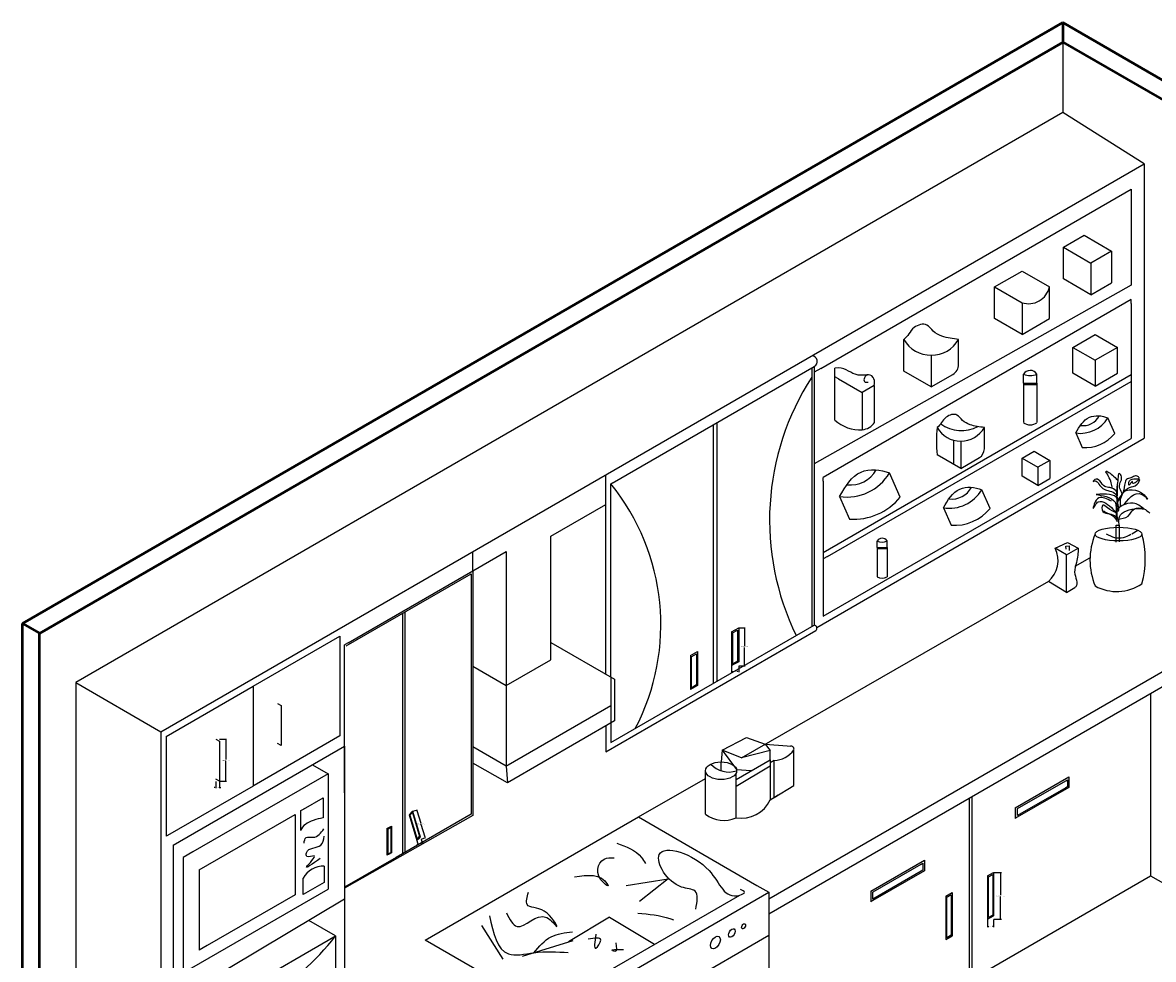
# Model space of a CAD drawing. Units: centimetres. Extents: x 5383 to 11288, y 5305 to 11515.
# Tile 3 of 5: x 5383 to 5675, y 5610 to 5851. Entities that reach past the tile are written whole.
import ezdxf

# ---------------------------------------------------------------- set-up
doc = ezdxf.new("R2010")
doc.units = ezdxf.units.CM
for name, color, linetype, lineweight in [('A-ANNO-DIMS', 2, 'Continuous', 18), ('A-EQPM', 4, 'Continuous', 25), ('A-FLOR-CASE', 3, 'Continuous', 25), ('A-WALL', 7, 'Continuous', 50)]:
    doc.layers.add(name, color=color, linetype=linetype, lineweight=lineweight)
doc.styles.get("Standard").update_dxf_attribs({"font": 'arial.ttf'})
doc.dimstyles.get("Standard").update_dxf_attribs({"dimtxt": 0.18, "dimasz": 0.18, "dimexe": 0.18, "dimexo": 0.0625, "dimgap": 0.09, "dimtad": 0, "dimtih": 1, "dimtoh": 1, "dimdec": 4, "dimzin": 0, "dimdsep": 46, "dimtxsty": 'Standard', "dimcen": 0.09, "dimadec": 0, "dimazin": 0, "dimtfac": 1, "dimtdec": 4, "dimtofl": 0, "dimtmove": 0, "dimatfit": 3, "dimfxl": 1, "dimtolj": 1, "dimtzin": 0, "dimarcsym": 0})

# ---------------------------------------------------------------- blocks, each defined once
blk = doc.blocks.new('HANDLE-DOOR-A')
for p, q in [((0, 8.75), (1.82, 9.8)), ((0.24, 8.46), (1.54, 9.21)), ((1.54, 9.21), (1.54, 1.19)), ((1.82, 9.8), (1.82, 1.05)), ((0, 8.75), (0, 0)), ((0.24, 8.46), (0.24, 0.44)), ((0.49, 0.29), (0, 0)), ((0.33, 0.49), (0.24, 0.44)), ((1.54, 1.19), (0.33, 0.49)), ((1.82, 1.05), (0.49, 0.29))]:
    blk.add_line(p, q)
blk = doc.blocks.new('HANDLE-DOOR-B')
for p, q in [((0, 6.88), (1.13, 7.53)), ((0, 6.88), (0, 0)), ((0.2, 6.74), (0.98, 7.19)), ((0.2, 6.74), (0.2, 0.29)), ((0.98, 7.19), (0.98, 0.75)), ((1.13, 7.53), (1.13, 0.65)), ((0.41, 0.24), (0, 0)), ((0.2, 0.29), (0.98, 0.75)), ((1.13, 0.65), (0.41, 0.24))]:
    blk.add_line(p, q)
blk = doc.blocks.new('HANDLE-DOOR-C')
for p, q in [((0, 11.18), (1.56, 12.08)), ((1.56, 12.08), (1.56, 0.91)), ((0, 11.18), (0, 0)), ((0.24, 10.92), (1.35, 11.56)), ((0.24, 0.46), (0.24, 10.92)), ((1.35, 11.56), (1.35, 1.1)), ((0, 0), (1.56, 0.91)), ((1.35, 1.1), (0.24, 0.46)), ((1.56, 0.91), (0.77, 0.45))]:
    blk.add_line(p, q)
blk = doc.blocks.new('HANDLE-DOOR-F')
for p, q in [((0, 10.85), (0.96, 10.3)), ((0.96, 10.3), (0.96, 0)), ((0.96, 0), (0, 0.55))]:
    blk.add_line(p, q)
blk = doc.blocks.new('*D18')
at = {"layer": 'A-ANNO-DIMS', "color": 0, "lineweight": -2, "transparency": 16777216}
for p, q in [((5567.7, 5695.2), (5569.28, 5695.2)), ((5569.1, 5695.02), (5569.1, 5690.48)), ((5569.1, 5685.57), (5569.1, 5690.11)), ((5567.7, 5685.39), (5569.28, 5685.39))]:
    blk.add_line(p, q, dxfattribs=at)
at = {"layer": 'A-ANNO-DIMS', "color": 0, "transparency": 16777216}
for points in [[(5569.07, 5695.02), (5569.13, 5695.02), (5569.1, 5695.2)], [(5569.07, 5685.57), (5569.13, 5685.57), (5569.1, 5685.39)]]:
    blk.add_solid(points, dxfattribs=at)
at = {"layer": 'Defpoints', "color": 0, "transparency": 16777216}
for p in [(5567.63, 5695.2), (5569.1, 5695.2), (5567.63, 5685.39)]:
    blk.add_point(p, dxfattribs=at)
at = {"layer": 'A-ANNO-DIMS', "color": 0, "transparency": 16777216, "insert": (5569.1, 5690.29), "char_height": 0.18, "attachment_point": 5}
blk.add_mtext('\\A1;HANDLE A 10 TYP.', dxfattribs=at)
blk = doc.blocks.new('*D19')
at = {"layer": 'A-ANNO-DIMS', "color": 0, "lineweight": -2, "transparency": 16777216}
for p, q in [((5565.81, 5685.33), (5565.81, 5683.74)), ((5567.63, 5685.33), (5567.63, 5683.74)), ((5565.99, 5683.92), (5566.26, 5683.92)), ((5567.45, 5683.92), (5567.18, 5683.92))]:
    blk.add_line(p, q, dxfattribs=at)
at = {"layer": 'A-ANNO-DIMS', "color": 0, "transparency": 16777216}
for points in [[(5565.99, 5683.95), (5565.99, 5683.89), (5565.81, 5683.92)], [(5567.45, 5683.95), (5567.45, 5683.89), (5567.63, 5683.92)]]:
    blk.add_solid(points, dxfattribs=at)
at = {"layer": 'Defpoints', "color": 0, "transparency": 16777216}
for p in [(5565.81, 5685.39), (5567.63, 5685.39), (5567.63, 5683.92)]:
    blk.add_point(p, dxfattribs=at)
at = {"layer": 'A-ANNO-DIMS', "color": 0, "transparency": 16777216, "insert": (5566.72, 5683.92), "char_height": 0.18, "attachment_point": 5}
blk.add_mtext('\\A1;2 TYP.', dxfattribs=at)
blk = doc.blocks.new('*D20')
at = {"layer": 'A-ANNO-DIMS', "color": 0, "lineweight": -2, "transparency": 16777216}
for p, q in [((5483.53, 5647.9), (5484.72, 5648.26)), ((5484.6, 5648.03), (5485.59, 5644.78)), ((5486.68, 5641.17), (5485.7, 5644.42)), ((5485.71, 5640.69), (5486.91, 5641.05))]:
    blk.add_line(p, q, dxfattribs=at)
at = {"layer": 'A-ANNO-DIMS', "color": 0, "transparency": 16777216}
for points in [[(5484.63, 5648.04), (5484.57, 5648.03), (5484.55, 5648.21)], [(5486.71, 5641.18), (5486.65, 5641.16), (5486.74, 5641)]]:
    blk.add_solid(points, dxfattribs=at)
at = {"layer": 'Defpoints', "color": 0, "transparency": 16777216}
for p in [(5483.47, 5647.88), (5484.55, 5648.21), (5485.65, 5640.67)]:
    blk.add_point(p, dxfattribs=at)
at = {"layer": 'A-ANNO-DIMS', "color": 0, "transparency": 16777216, "insert": (5485.64, 5644.6), "char_height": 0.18, "attachment_point": 5}
blk.add_mtext('\\A1;HANDLE B 8 TYP.', dxfattribs=at)
blk = doc.blocks.new('*D21')
at = {"layer": 'A-ANNO-DIMS', "color": 0, "lineweight": -2, "transparency": 16777216}
for p, q in [((5484.73, 5639.21), (5484.55, 5639.15)), ((5484.59, 5640.28), (5484.95, 5639.09)), ((5485.67, 5640.61), (5486.03, 5639.41)), ((5486.15, 5639.64), (5486.33, 5639.69))]:
    blk.add_line(p, q, dxfattribs=at)
at = {"layer": 'A-ANNO-DIMS', "color": 0, "transparency": 16777216}
for points in [[(5484.72, 5639.23), (5484.73, 5639.18), (5484.9, 5639.26)], [(5486.15, 5639.67), (5486.16, 5639.61), (5485.98, 5639.59)]]:
    blk.add_solid(points, dxfattribs=at)
at = {"layer": 'Defpoints', "color": 0, "transparency": 16777216}
for p in [(5484.57, 5640.34), (5485.65, 5640.67), (5485.98, 5639.59)]:
    blk.add_point(p, dxfattribs=at)
at = {"layer": 'A-ANNO-DIMS', "color": 0, "transparency": 16777216, "insert": (5485.44, 5639.42), "char_height": 0.18, "attachment_point": 5}
blk.add_mtext('\\A1;1 TYP.', dxfattribs=at)
blk = doc.blocks.new('*D22')
at = {"layer": 'A-ANNO-DIMS', "color": 0, "lineweight": -2, "transparency": 16777216}
for p, q in [((5633.49, 5632.05), (5635.42, 5632.05)), ((5635.24, 5631.87), (5635.24, 5626.2)), ((5635.24, 5620.16), (5635.24, 5625.83)), ((5633.49, 5619.98), (5635.42, 5619.98))]:
    blk.add_line(p, q, dxfattribs=at)
at = {"layer": 'A-ANNO-DIMS', "color": 0, "transparency": 16777216}
for points in [[(5635.21, 5631.87), (5635.27, 5631.87), (5635.24, 5632.05)], [(5635.21, 5620.16), (5635.27, 5620.16), (5635.24, 5619.98)]]:
    blk.add_solid(points, dxfattribs=at)
at = {"layer": 'Defpoints', "color": 0, "transparency": 16777216}
for p in [(5633.43, 5632.05), (5635.24, 5632.05), (5633.43, 5619.98)]:
    blk.add_point(p, dxfattribs=at)
at = {"layer": 'A-ANNO-DIMS', "color": 0, "transparency": 16777216, "insert": (5635.24, 5626.01), "char_height": 0.18, "attachment_point": 5}
blk.add_mtext('\\A1;HANDLE C 12 TYP.', dxfattribs=at)
blk = doc.blocks.new('*D23')
at = {"layer": 'A-ANNO-DIMS', "color": 0, "lineweight": -2, "transparency": 16777216}
for p, q in [((5631.87, 5619.91), (5631.87, 5617.98)), ((5632.05, 5618.16), (5632.19, 5618.16)), ((5633.25, 5618.16), (5633.11, 5618.16)), ((5633.43, 5619.91), (5633.43, 5617.98))]:
    blk.add_line(p, q, dxfattribs=at)
at = {"layer": 'A-ANNO-DIMS', "color": 0, "transparency": 16777216}
for points in [[(5632.05, 5618.19), (5632.05, 5618.13), (5631.87, 5618.16)], [(5633.25, 5618.19), (5633.25, 5618.13), (5633.43, 5618.16)]]:
    blk.add_solid(points, dxfattribs=at)
at = {"layer": 'Defpoints', "color": 0, "transparency": 16777216}
for p in [(5631.87, 5619.98), (5633.43, 5619.98), (5633.43, 5618.16)]:
    blk.add_point(p, dxfattribs=at)
at = {"layer": 'A-ANNO-DIMS', "color": 0, "transparency": 16777216, "insert": (5632.65, 5618.16), "char_height": 0.18, "attachment_point": 5}
blk.add_mtext('\\A1;2 TYP.', dxfattribs=at)
blk = doc.blocks.new('*D30')
at = {"layer": 'A-ANNO-DIMS', "color": 0, "lineweight": -2, "transparency": 16777216}
for p, q in [((5433.68, 5666.45), (5435.42, 5666.45)), ((5435.24, 5666.27), (5435.24, 5661.2)), ((5435.24, 5655.77), (5435.24, 5660.84)), ((5433.68, 5655.59), (5435.42, 5655.59))]:
    blk.add_line(p, q, dxfattribs=at)
at = {"layer": 'A-ANNO-DIMS', "color": 0, "transparency": 16777216}
for points in [[(5435.21, 5666.27), (5435.27, 5666.27), (5435.24, 5666.45)], [(5435.21, 5655.77), (5435.27, 5655.77), (5435.24, 5655.59)]]:
    blk.add_solid(points, dxfattribs=at)
at = {"layer": 'Defpoints', "color": 0, "transparency": 16777216}
for p in [(5433.61, 5666.45), (5435.24, 5666.45), (5433.61, 5655.59)]:
    blk.add_point(p, dxfattribs=at)
at = {"layer": 'A-ANNO-DIMS', "color": 0, "transparency": 16777216, "insert": (5435.24, 5661.02), "char_height": 0.18, "attachment_point": 5}
blk.add_mtext('\\A1;HANDLE F 11 TYP.', dxfattribs=at)
blk = doc.blocks.new('*D31')
at = {"layer": 'A-ANNO-DIMS', "color": 0, "lineweight": -2, "transparency": 16777216}
for p, q in [((5432.48, 5653.97), (5432.3, 5653.97)), ((5432.66, 5655.53), (5432.66, 5653.79)), ((5433.61, 5655.53), (5433.61, 5653.79)), ((5433.79, 5653.97), (5433.97, 5653.97))]:
    blk.add_line(p, q, dxfattribs=at)
at = {"layer": 'A-ANNO-DIMS', "color": 0, "transparency": 16777216}
for points in [[(5432.48, 5654), (5432.48, 5653.94), (5432.66, 5653.97)], [(5433.79, 5654), (5433.79, 5653.94), (5433.61, 5653.97)]]:
    blk.add_solid(points, dxfattribs=at)
at = {"layer": 'Defpoints', "color": 0, "transparency": 16777216}
for p in [(5432.66, 5655.59), (5433.61, 5655.59), (5433.61, 5653.97)]:
    blk.add_point(p, dxfattribs=at)
at = {"layer": 'A-ANNO-DIMS', "color": 0, "transparency": 16777216, "insert": (5433.14, 5653.97), "char_height": 0.18, "attachment_point": 5}
blk.add_mtext('\\A1;1 TYP.', dxfattribs=at)

msp = doc.modelspace()

# ---------------------------------------------------------------- linework, layer by layer
at = {"layer": 'A-EQPM'}
for p, q in [((5533.38, 5683.19), (5533.38, 5734.67)), ((5519.18, 5718.86), (5533.38, 5727.01)), ((5519.18, 5686.95), (5519.18, 5718.86)), ((5499.05, 5685.25), (5507.64, 5680.29)), ((5507.64, 5680.29), (5519.18, 5686.95)), ((5457.63, 5659.86), (5461.66, 5657.53)), ((5461.66, 5657.53), (5426.73, 5637.37)), ((5461.66, 5657.53), (5461.66, 5627.75)), ((5541.77, 5646.4), (5559.1, 5656.34)), ((5455.31, 5648.43), (5460.36, 5651.35)), ((5460.36, 5651.35), (5460.36, 5646.17)), ((5428.43, 5632.72), (5453.15, 5647)), ((5453.15, 5647), (5453.15, 5626.31)), ((5454.67, 5648.08), (5455.89, 5648.77)), ((5454.67, 5642.89), (5454.67, 5648.08)), ((5486.72, 5614.62), (5541.77, 5646.4)), ((5541.77, 5646.4), (5572.35, 5628.74)), ((5426.73, 5637.37), (5424.24, 5635.93)), ((5424.24, 5635.93), (5424.24, 5606.15)), ((5428.43, 5632.72), (5428.43, 5612.23)), ((5460.68, 5633.67), (5460.68, 5629.48)), ((5455.24, 5626.34), (5455.24, 5630.57)), ((5460.68, 5629.48), (5455.24, 5626.34)), ((5538.63, 5628.74), (5549.42, 5630.41)), ((5549.42, 5630.41), (5542.07, 5624.55)), ((5424.24, 5606.15), (5461.66, 5627.75)), ((5520.4, 5595.18), (5575.44, 5626.96)), ((5572.35, 5628.74), (5575.44, 5626.96)), ((5575.44, 5626.96), (5575.44, 5615.8)), ((5465.93, 5625.19), (5424.24, 5600.32)), ((5453.15, 5626.31), (5430.43, 5613.2)), ((5520.3, 5598.74), (5567.93, 5626.24)), ((5501.25, 5618.39), (5506.79, 5609.7)), ((5534.29, 5620.52), (5523.7, 5614.15)), ((5534.29, 5620.52), (5545.94, 5613.54)), ((5575.44, 5615.8), (5520.4, 5584.02)), ((5575.44, 5615.8), (5575.44, 5574.33)), ((5430.43, 5613.2), (5428.43, 5612.04)), ((5428.43, 5612.23), (5428.43, 5612.04)), ((5520.4, 5595.18), (5486.72, 5614.62)), ((5511.85, 5610.43), (5524.88, 5614.52))]:
    msp.add_line(p, q, dxfattribs=at)
msp.add_arc((5460.45, 5627.75), 5.93, 87.7657, 151.5311, dxfattribs=at)
for centre, major_axis in [((5565.87, 5616.43), (-0.61, -1.05)), ((5568.89, 5618.17), (-0.368, -0.638)), ((5561.63, 5613.98), (-0.9, -1.55))]:
    msp.add_ellipse(centre, major_axis=major_axis, ratio=0.57735, dxfattribs=at)
for points, knots in [([(5460.36, 5646.17), (5459.55, 5645.98), (5457.46, 5645.48), (5454.9, 5644.17), (5454.67, 5642.89)], [0, 0, 0, 0, 2.608233, 6.700151, 6.700151, 6.700151, 6.700151]), ([(5455.46, 5639.64), (5455.55, 5640.23), (5455.74, 5641.55), (5458.64, 5640.66), (5459.81, 5642.24), (5460.58, 5643.29)], [0, 0, 0, 0, 1.518182, 3.345478, 6.853378, 6.853378, 6.853378, 6.853378]), ([(5459.63, 5635.68), (5457.66, 5634.26), (5454.08, 5631.68), (5459.75, 5637.33), (5456.02, 5635.56), (5455.97, 5638.7), (5460.16, 5638.07), (5460.53, 5640.51), (5460.66, 5641.39)], [0, 0, 0, 0, 4.047225, 7.363085, 9.194771, 10.155201, 14.385132, 16.797476, 16.797476, 16.797476, 16.797476]), ([(5536.16, 5639.64), (5538.6, 5638.74), (5541.66, 5637.6), (5543.28, 5634.92), (5543.61, 5634.37)], [0, 0, 0, 0, 7.386801, 9.288551, 9.288551, 9.288551, 9.288551]), ([(5556.55, 5622.59), (5556.9, 5624.51), (5557.53, 5627.95), (5550.15, 5627.71), (5542.48, 5641.3), (5561.88, 5634.99), (5563.87, 5624.44), (5569.7, 5626.92), (5568.59, 5627.4), (5568.06, 5627.63)], [0, 0, 0, 0, 4.660279, 8.330693, 18.454163, 31.926211, 42.090752, 43.472118, 44.746413, 44.746413, 44.746413, 44.746413]), ([(5525.26, 5630.95), (5528.64, 5631.44), (5532.15, 5631.95), (5534.19, 5628.29), (5530.22, 5630.93), (5531.43, 5635.96), (5534.57, 5635.86), (5535.49, 5635.83)], [0, 0, 0, 0, 8.778444, 9.119705, 10.35063, 16.607257, 19.221094, 19.221094, 19.221094, 19.221094]), ([(5507.7, 5621.64), (5508.52, 5620), (5510.81, 5615.44), (5516.6, 5623.49), (5522.14, 5615.93), (5517.91, 5623.64), (5512.18, 5622.55), (5513.01, 5625.7), (5513.35, 5626.98)], [0, 0, 0, 0, 4.458018, 12.428882, 15.889863, 20.991355, 25.727205, 28.946338, 28.946338, 28.946338, 28.946338]), ([(5503.3, 5620.84), (5504.28, 5616.44), (5505.84, 5609.41), (5515.77, 5611.86), (5520.76, 5611.59), (5523.63, 5611.43)], [0, 0, 0, 0, 10.970099, 17.518453, 26.404777, 26.404777, 26.404777, 26.404777]), ([(5541.63, 5621.58), (5544.43, 5621.32), (5547.56, 5621.02), (5550.49, 5619.94), (5550.79, 5619.83)], [0, 0, 0, 0, 8.376196, 9.342218, 9.342218, 9.342218, 9.342218]), ([(5514.75, 5611.34), (5516.12, 5612.94), (5518.76, 5616.03), (5522.79, 5616.51), (5524.73, 5616.74)], [0, 0, 0, 0, 6.070874, 11.732161, 11.732161, 11.732161, 11.732161]), ([(5530.79, 5616.12), (5530.48, 5614.19), (5529.95, 5610.97), (5533.21, 5615.63), (5530.4, 5615.15), (5528.77, 5614.87)], [0, 0, 0, 0, 3.555518, 5.929323, 9.211396, 9.211396, 9.211396, 9.211396]), ([(5535.89, 5613.88), (5536.13, 5612.78), (5536.44, 5611.35), (5534.05, 5612.23), (5536.17, 5612.2), (5537.9, 5612.17)], [0, 0, 0, 0, 2.20234, 2.83923, 5.661966, 5.661966, 5.661966, 5.661966])]:
    msp.add_open_spline(points, degree=3, knots=knots, dxfattribs=at)
at = {"layer": 'A-FLOR-CASE'}
for p, q in [((5651.3, 5846.21), (5651.3, 5828.15)), ((5651.3, 5828.15), (5396.53, 5681.06)), ((5672.32, 5814.89), (5651.3, 5828.15)), ((5418.53, 5668.36), (5672.32, 5814.89)), ((5672.32, 5814.89), (5672.32, 5744.1)), ((5588.84, 5762.08), (5668.92, 5808.32)), ((5668.92, 5808.32), (5668.92, 5783.56)), ((5651.42, 5793.36), (5656.79, 5796.47)), ((5656.78, 5796.47), (5663.86, 5792.39)), ((5651.42, 5785.19), (5651.42, 5793.36)), ((5651.42, 5793.36), (5658.49, 5789.28)), ((5663.87, 5792.38), (5658.49, 5789.28)), ((5663.86, 5792.39), (5663.87, 5792.38)), ((5663.87, 5792.38), (5663.87, 5784.21)), ((5633.69, 5783.13), (5640.76, 5787.21)), ((5640.76, 5787.21), (5647.84, 5783.13)), ((5658.49, 5789.28), (5658.49, 5781.11)), ((5658.49, 5781.11), (5651.42, 5785.19)), ((5658.49, 5781.11), (5663.87, 5784.21)), ((5668.92, 5783.56), (5587.15, 5737.46)), ((5633.69, 5774.96), (5633.69, 5783.13)), ((5633.69, 5783.13), (5640.76, 5779.04)), ((5647.84, 5774.96), (5647.84, 5783.13)), ((5668.92, 5779.91), (5589.43, 5734.01)), ((5640.76, 5779.04), (5640.76, 5770.87)), ((5668.92, 5778.88), (5668.92, 5779.91)), ((5668.92, 5778.88), (5668.92, 5760.43)), ((5640.76, 5770.87), (5633.69, 5774.96)), ((5640.76, 5770.87), (5647.84, 5774.96)), ((5610.24, 5761.42), (5610.24, 5769.59)), ((5624.4, 5763.15), (5624.4, 5769.59)), ((5653.91, 5767.52), (5659.66, 5770.84)), ((5659.66, 5770.84), (5665.41, 5767.52)), ((5653.91, 5760.88), (5653.91, 5767.52)), ((5653.91, 5767.52), (5659.66, 5764.2)), ((5665.41, 5767.52), (5659.66, 5764.2)), ((5665.41, 5760.88), (5665.41, 5767.52)), ((5617.32, 5765.51), (5617.32, 5757.33)), ((5659.66, 5764.2), (5659.66, 5757.57)), ((5535.01, 5732.54), (5587.15, 5762.65)), ((5586.52, 5762.28), (5586.52, 5695.51)), ((5587.15, 5762.65), (5587.15, 5695.88)), ((5588.84, 5762.08), (5587.15, 5761.11)), ((5592.48, 5748.74), (5592.48, 5762.17)), ((5617.32, 5757.33), (5610.24, 5761.42)), ((5644.62, 5758.32), (5644.62, 5760.67)), ((5659.66, 5757.57), (5653.91, 5760.88)), ((5659.66, 5757.57), (5665.41, 5760.88)), ((5668.92, 5760.43), (5589.43, 5714.53)), ((5590.52, 5713.61), (5668.92, 5758.75)), ((5593.39, 5759.41), (5592.48, 5759.93)), ((5593.39, 5759.41), (5599.52, 5755.93)), ((5617.32, 5757.33), (5622.9, 5760.55)), ((5641.11, 5758.32), (5641.11, 5760.61)), ((5641.11, 5758.32), (5641.11, 5748.12)), ((5641.11, 5758.32), (5644.62, 5758.32)), ((5641.11, 5758), (5644.62, 5758)), ((5644.62, 5758.32), (5644.62, 5748.12)), ((5668.92, 5760.43), (5668.92, 5744.07)), ((5602.58, 5757.7), (5599.52, 5755.93)), ((5599.52, 5755.93), (5599.52, 5746.29)), ((5602.71, 5748.16), (5602.71, 5757.7)), ((5664.7, 5745.34), (5662.92, 5749.38)), ((5561.08, 5747.6), (5561.08, 5680.83)), ((5561.98, 5748.12), (5561.98, 5681.35)), ((5631.04, 5741.33), (5631.04, 5746.87)), ((5587.77, 5695.29), (5672.32, 5744.1)), ((5589.43, 5698.17), (5668.92, 5744.07)), ((5623.11, 5743.6), (5623.11, 5737.37)), ((5624.94, 5743.35), (5624.94, 5736.31)), ((5654.61, 5745.45), (5656.27, 5741.69)), ((5640.78, 5738.95), (5643.85, 5740.72)), ((5643.85, 5740.72), (5647.9, 5738.39)), ((5624.94, 5736.31), (5618.85, 5739.83)), ((5624.94, 5736.31), (5629.75, 5739.09)), ((5640.78, 5734.27), (5640.78, 5738.95)), ((5640.78, 5738.95), (5644.83, 5736.61)), ((5647.9, 5738.38), (5644.83, 5736.61)), ((5647.9, 5738.38), (5647.9, 5733.71)), ((5609.34, 5728.9), (5606.58, 5735.16)), ((5644.83, 5736.61), (5644.83, 5731.94)), ((5535.01, 5732.54), (5534.64, 5732.33)), ((5534.64, 5730.09), (5534.64, 5732.33)), ((5589.43, 5732.98), (5589.43, 5734.01)), ((5589.43, 5732.98), (5589.43, 5698.17)), ((5644.83, 5731.94), (5640.78, 5734.27)), ((5644.83, 5731.94), (5647.9, 5733.71)), ((5665.32, 5722.65), (5665.32, 5731.74)), ((5534.64, 5682.45), (5534.64, 5730.09)), ((5593.68, 5729.07), (5596.26, 5723.24)), ((5632.5, 5726), (5630.38, 5730.82)), ((5620.45, 5726.14), (5622.44, 5721.64)), ((5665.04, 5717.29), (5665.04, 5721.65)), ((5665.04, 5721.65), (5665.95, 5721.65)), ((5665.95, 5717.35), (5665.95, 5721.65)), ((5669.07, 5719.45), (5670.67, 5720.37)), ((5603.34, 5715.92), (5603.34, 5717.61)), ((5605.93, 5715.89), (5605.93, 5717.61)), ((5649.34, 5715.7), (5652.5, 5717.18)), ((5652.5, 5717.18), (5655.25, 5715.75)), ((5499.05, 5709.91), (5507.64, 5714.88)), ((5499.05, 5709.91), (5499.05, 5714.85)), ((5507.64, 5714.88), (5507.64, 5669.22)), ((5603.36, 5715.89), (5603.36, 5708.38)), ((5603.36, 5715.89), (5605.93, 5715.89)), ((5603.36, 5715.65), (5605.93, 5715.65)), ((5605.93, 5715.89), (5605.93, 5708.38)), ((5652.25, 5714.02), (5649.34, 5715.7)), ((5652.04, 5716.28), (5652.92, 5716.35)), ((5652.11, 5715.47), (5652.04, 5716.28)), ((5652.25, 5714.02), (5655.25, 5715.75)), ((5652.25, 5704.32), (5652.25, 5714.02)), ((5652.92, 5716.35), (5652.92, 5715.12)), ((5590.52, 5713.61), (5589.43, 5712.97)), ((5654.5, 5711.09), (5658.29, 5713.27)), ((5466.33, 5690.51), (5498.59, 5709.14)), ((5466.82, 5691.3), (5499.05, 5709.91)), ((5498.59, 5709.14), (5498.59, 5647.1)), ((5499.05, 5709.91), (5499.05, 5646.79)), ((5568.34, 5661.65), (5647.69, 5707.18)), ((5652.25, 5704.32), (5647.57, 5707.13)), ((5652.25, 5704.32), (5654.39, 5705.55)), ((5480.84, 5698.89), (5480.84, 5636.85)), ((5481.5, 5699.27), (5481.5, 5637.23)), ((5533.38, 5663.18), (5587.57, 5694.46)), ((5534.64, 5665.56), (5587.15, 5695.88)), ((5442.33, 5680.13), (5464.69, 5693.05)), ((5464.69, 5693.05), (5464.69, 5667.28)), ((5466.82, 5691.3), (5465.93, 5690.79)), ((5465.93, 5690.43), (5465.93, 5690.79)), ((5519.18, 5691.38), (5535.6, 5681.9)), ((5465.93, 5687.71), (5465.93, 5690.43)), ((5465.93, 5652.59), (5465.93, 5687.71)), ((5575.44, 5625.3), (5678.79, 5684.97)), ((5534.64, 5682.45), (5534.64, 5665.56)), ((5535.6, 5681.9), (5535.6, 5675.63)), ((5396.53, 5681.06), (5396.53, 5496.36)), ((5396.53, 5681.06), (5418.53, 5668.36)), ((5419.92, 5667.17), (5442.29, 5680.09)), ((5442.29, 5680.09), (5442.29, 5654.32)), ((5442.33, 5680.13), (5442.33, 5654.37)), ((5575.44, 5621.38), (5678.79, 5681.05)), ((5673.95, 5678.25), (5673.95, 5631.2)), ((5534.64, 5675.07), (5508.13, 5659.77)), ((5535.6, 5675.63), (5535.6, 5671.17)), ((5535.6, 5671.17), (5507.93, 5655.19)), ((5418.53, 5668.36), (5418.53, 5504.61)), ((5464.69, 5667.28), (5442.61, 5654.53)), ((5507.64, 5669.22), (5507.64, 5659.48)), ((5533.38, 5669.88), (5533.38, 5663.18)), ((5419.92, 5667.17), (5419.92, 5641.41)), ((5421.66, 5639.1), (5465.93, 5664.66)), ((5465.93, 5664.66), (5465.93, 5511.54)), ((5507.64, 5659.48), (5499.05, 5664.45)), ((5563.37, 5663.6), (5569.64, 5666.91)), ((5569.64, 5666.91), (5574.47, 5665.17)), ((5574.47, 5665.17), (5575.77, 5663.5)), ((5574.47, 5665.17), (5580.17, 5664.7)), ((5580.17, 5664.7), (5580.98, 5664.63)), ((5563.37, 5663.6), (5563.1, 5660.59)), ((5568.34, 5661.65), (5563.37, 5663.6)), ((5563.37, 5663.6), (5567.07, 5658.61)), ((5575.77, 5663.5), (5568.34, 5661.65)), ((5575.77, 5661.16), (5575.77, 5663.5)), ((5575.77, 5663.5), (5575.77, 5663.5)), ((5581.88, 5654.5), (5581.88, 5663.7)), ((5507.93, 5655.19), (5499.05, 5660.27)), ((5508.13, 5659.77), (5507.64, 5659.48)), ((5507.64, 5659.48), (5507.93, 5655.19)), ((5563.1, 5658.31), (5563.1, 5660.59)), ((5565.6, 5660.07), (5565.61, 5660.08)), ((5566.96, 5656.07), (5575.77, 5661.16)), ((5575.77, 5659.46), (5566.96, 5654.22)), ((5567.07, 5658.61), (5570.89, 5658.34)), ((5575.77, 5661.16), (5575.77, 5659.46)), ((5576.79, 5660.92), (5575.77, 5660.31)), ((5575.77, 5659.46), (5575.77, 5650.81)), ((5576.79, 5651.43), (5576.79, 5660.92)), ((5559.1, 5654.15), (5559.1, 5658.2)), ((5566.96, 5646.18), (5566.96, 5657.69)), ((5638.98, 5648.74), (5652.83, 5656.73)), ((5639.63, 5648.55), (5652.02, 5655.7)), ((5652.02, 5655.7), (5652.47, 5655.96)), ((5652.47, 5655.96), (5652.47, 5654.18)), ((5652.83, 5656.73), (5652.83, 5654)), ((5442.29, 5654.32), (5420.2, 5641.57)), ((5442.61, 5654.53), (5442.29, 5654.32)), ((5559.1, 5647.14), (5559.1, 5654.15)), ((5576.79, 5651.43), (5581.88, 5654.5)), ((5652.83, 5654), (5639.54, 5646.33)), ((5652.02, 5653.92), (5639.56, 5646.72)), ((5652.47, 5654.18), (5652.02, 5653.92)), ((5575.77, 5650.81), (5577.82, 5652.05)), ((5627.11, 5651.21), (5627.11, 5604.16)), ((5627.78, 5651.6), (5627.78, 5604.55)), ((5498.59, 5647.1), (5479.26, 5635.94)), ((5638.98, 5648.74), (5638.98, 5646.01)), ((5639.56, 5646.72), (5639.56, 5648.51)), ((5499.05, 5646.79), (5465.93, 5628.03)), ((5639.54, 5646.33), (5638.98, 5646.01)), ((5420.2, 5641.57), (5419.92, 5641.41)), ((5421.66, 5639.1), (5421.66, 5485.47)), ((5479.26, 5635.94), (5465.93, 5628.25)), ((5601.71, 5627.22), (5615.55, 5635.21)), ((5615.55, 5635.21), (5615.55, 5632.48)), ((5615.55, 5632.48), (5602.27, 5624.81)), ((5614.74, 5632.4), (5602.29, 5625.2)), ((5602.35, 5627.03), (5614.74, 5634.18)), ((5614.74, 5634.18), (5615.19, 5634.44)), ((5615.19, 5632.65), (5614.74, 5632.4)), ((5615.19, 5634.44), (5615.19, 5632.65)), ((5558.33, 5564.45), (5673.95, 5631.2)), ((5673.95, 5631.2), (5736.51, 5595.08)), ((5601.71, 5627.22), (5601.71, 5624.49)), ((5602.35, 5627.03), (5602.29, 5626.99)), ((5602.29, 5625.2), (5602.29, 5626.99)), ((5602.27, 5624.81), (5601.71, 5624.49)), ((5463.6, 5615.69), (5456.7, 5619.68)), ((5461.72, 5614.61), (5463.6, 5615.69)), ((5463.6, 5615.69), (5463.6, 5518.14)), ((5421.66, 5591.48), (5461.72, 5614.61))]:
    msp.add_line(p, q, dxfattribs=at)
for centre, radius, start, end in [((5642.41, 5784.36), 5.56, 252.7563, 347.2437), ((5617.32, 5773.68), 8.17, 210, 330), ((5586.43, 5763.93), 1.47, 299.3685, 84.2474), ((5621.4, 5763.15), 3, 300, 0), ((5642.88, 5759.53), 2.07, 33.2806, 148.588), ((5642.8, 5764.51), 4.25, 246.6072, 295.2614), ((5643.44, 5722.98), 67.84, 147.0474, 206.05), ((5655.84, 5753.61), 8.25, 261.3996, 329.1091), ((5656.51, 5752.1), 4.74, 261.8793, 332.0456), ((5598.95, 5756.04), 9.76, 228.4196, 273.3124), ((5599.15, 5750.59), 4.31, 274.8828, 325.6975), ((5650.2, 5743.35), 31.55, 173.5951, 186.4049), ((5624.94, 5750.39), 7.04, 210, 330), ((5625.17, 5755.01), 8.97, 233.0487, 298.0753), ((5642.86, 5750.61), 3.05, 234.9464, 305.0536), ((5656.95, 5751.69), 10.02, 266.1295, 320.698), ((5628.45, 5741.33), 2.58, 300, 0), ((5595.59, 5741.73), 12.8, 261.3996, 329.1091), ((5596.62, 5739.39), 7.35, 261.8793, 332.0456), ((5489.88, 5695.98), 57.67, 332.3397, 39.0788), ((5597.3, 5738.75), 15.55, 266.1295, 320.698), ((5621.93, 5735.87), 9.85, 261.3996, 329.1091), ((5622.71, 5734.07), 5.65, 261.8793, 332.0456), ((5623.24, 5733.58), 11.96, 266.1295, 320.698), ((5604.66, 5716.77), 1.52, 33.2806, 148.588), ((5604.6, 5720.44), 3.13, 246.6072, 295.2614), ((5675.57, 5712.68), 17.28, 157.2197, 202.7803), ((5647.6, 5712.96), 24.95, 345.1121, 14.8879), ((5642.82, 5712.58), 7.23, 311.0571, 25.5985), ((5604.64, 5710.21), 2.24, 234.9464, 305.0536), ((5665.21, 5716.12), 11.57, 241.172, 304.1782), ((5586.95, 5695.05), 0.852, 316.2625, 76.2625), ((5426.4, 5631.7), 40.5, 66.8388, 66.9018), ((5581.17, 5663.91), 0.745, 343.4856, 104.3086), ((5576.44, 5667.62), 6.71, 273.0044, 324.1801), ((5565.07, 5664.27), 6.3, 222.5539, 288.8818), ((5568.38, 5654.19), 8.13, 259.939, 335.4526), ((5563.78, 5652.86), 7.39, 230.6657, 295.4474), ((5413.21, 5654.54), 63.63, 277.6292, 322.3708)]:
    msp.add_arc(centre, radius, start, end, dxfattribs=at)
for centre, major_axis, ratio in [((5665.67, 5719.37), (-6.04, 0), 0.292852), ((5563.1, 5658.31), (-4.01, 0), 0.569076)]:
    msp.add_ellipse(centre, major_axis=major_axis, ratio=ratio, dxfattribs=at)
for points, knots in [([(5624.4, 5769.59), (5622.94, 5769.77), (5620.61, 5770.04), (5617.79, 5771.47), (5616.2, 5774.03), (5612.17, 5772.94), (5611.31, 5770.29), (5610.24, 5769.59)], [0, 0, 0, 0, 4.38311, 6.972047, 9.273965, 12.593909, 16.675124, 16.675124, 16.675124, 16.675124]), ([(5600.87, 5760.41), (5599.79, 5760.34), (5597.07, 5760.14), (5594.76, 5762.58), (5592.48, 5762.17)], [0, 0, 0, 0, 2.115163, 5.365679, 5.365679, 5.365679, 5.365679]), ([(5602.58, 5757.7), (5602.68, 5758.28), (5602.88, 5759.46), (5601.26, 5760.91), (5599.96, 5759.91), (5599.87, 5758.47), (5600.67, 5758.53), (5601.09, 5758.56)], [0, 0, 0, 0, 1.692298, 3.480179, 4.827654, 5.771982, 6.812324, 6.812324, 6.812324, 6.812324]), ([(5631.04, 5746.87), (5629.78, 5747.02), (5627.78, 5747.26), (5625.35, 5748.49), (5623.98, 5750.7), (5620.51, 5749.76), (5619.76, 5747.48), (5618.85, 5746.87)], [0, 0, 0, 0, 4.38311, 6.972047, 9.273965, 12.593909, 16.675124, 16.675124, 16.675124, 16.675124]), ([(5654.61, 5745.45), (5655.6, 5747.14), (5657.46, 5750.31), (5661.42, 5749.96), (5662.92, 5749.38)], [0, 0, 0, 0, 9.319983, 17.514468, 17.514468, 17.514468, 17.514468]), ([(5593.68, 5729.07), (5595.21, 5731.69), (5598.1, 5736.61), (5604.24, 5736.06), (5606.58, 5735.16)], [0, 0, 0, 0, 9.319983, 17.514468, 17.514468, 17.514468, 17.514468]), ([(5664.06, 5731.19), (5663.92, 5732.11), (5663.72, 5733.4), (5661.94, 5736.08), (5663.91, 5734.8), (5664.19, 5734.39), (5665.81, 5733.06), (5665.44, 5733.11), (5665.44, 5733.11)], [0, 0, 0, 0, 3.355351, 4.71948, 5.889388, 7.594456, 8.683008, 8.698185, 8.698185, 8.698185, 8.698185]), ([(5666.6, 5729.67), (5667.19, 5730.42), (5668.25, 5731.77), (5670.3, 5731.43), (5671.5, 5733.94), (5670.56, 5733.04), (5670.08, 5732.76), (5669.2, 5732.04), (5669.34, 5733.54), (5668.21, 5731.15), (5668.28, 5734.41), (5671.79, 5733.09), (5670.42, 5734.6), (5669.48, 5734.15), (5668.58, 5733.77), (5667.53, 5733.5), (5667.35, 5732.66), (5667.08, 5731.48), (5666.99, 5729.51), (5664.67, 5728.13), (5666.15, 5725.22), (5665.28, 5725.23), (5665.27, 5725.23)], [0, 0, 0, 0, 2.592905, 4.695293, 6.095645, 6.835537, 7.225482, 8.155293, 8.629482, 9.852059, 10.914667, 13.551571, 14.266731, 15.244139, 16.306784, 17.42104, 18.021399, 18.727344, 21.143013, 23.418353, 25.91724, 25.97222, 25.97222, 25.97222, 25.97222]), ([(5665.42, 5727.73), (5665.74, 5728.07), (5666.25, 5728.63), (5666.86, 5729.92), (5665.67, 5731.06), (5666.05, 5732.72), (5666.72, 5733.88), (5665.63, 5735.64), (5665.5, 5733.18), (5665.29, 5732.04), (5665.33, 5730.5), (5665.32, 5729.66), (5665.32, 5729.21)], [0, 0, 0, 0, 1.405563, 2.306551, 3.890673, 5.45856, 6.952379, 7.99153, 9.425529, 11.327143, 12.488132, 13.85322, 13.85322, 13.85322, 13.85322]), ([(5620.45, 5726.14), (5621.64, 5728.15), (5623.86, 5731.93), (5628.58, 5731.51), (5630.38, 5730.82)], [0, 0, 0, 0, 9.319983, 17.514468, 17.514468, 17.514468, 17.514468]), ([(5665.32, 5728.4), (5665.33, 5728.55), (5665.36, 5729.13), (5664.61, 5730.26), (5662.55, 5730.58), (5660.79, 5731.48), (5660.02, 5733.41), (5658.83, 5732.73), (5659.82, 5733.91), (5661.09, 5732.95), (5661.82, 5731.52), (5663.6, 5731.44), (5665.46, 5730.64), (5665.37, 5729.19), (5665.32, 5728.4)], [0, 0, 0, 0, 0.437629, 1.734716, 3.555033, 6.409331, 7.743531, 8.257448, 8.951242, 10.248329, 12.152328, 13.538735, 15.327436, 17.459929, 17.459929, 17.459929, 17.459929]), ([(5663.89, 5727.85), (5662.68, 5728.45), (5660.73, 5729.41), (5659.5, 5727.69), (5658.92, 5725.5), (5659.72, 5727.02), (5661.03, 5728.59), (5663.68, 5726.53), (5665.18, 5724.78), (5665.27, 5723.8), (5665.32, 5723.27)], [0, 0, 0, 0, 3.386527, 5.468894, 6.555678, 7.444372, 8.770788, 12.948194, 14.273332, 15.806246, 15.806246, 15.806246, 15.806246]), ([(5665.32, 5726.34), (5665.41, 5727.1), (5665.75, 5729.91), (5662.36, 5729.72), (5659.89, 5729.59)], [0, 0, 0, 0, 2.062076, 7.621415, 7.621415, 7.621415, 7.621415]), ([(5659.89, 5729.59), (5660.73, 5729.45), (5662.44, 5729.16), (5665.46, 5727.81), (5664.84, 5724.85), (5665.19, 5723.26), (5665.32, 5722.65)], [0, 0, 0, 0, 2.620458, 5.363994, 8.430173, 10.317804, 10.317804, 10.317804, 10.317804]), ([(5666.15, 5726.47), (5666.15, 5727.98), (5666.17, 5731.76), (5672.08, 5730.67), (5672.89, 5728.54), (5673.01, 5728.41)], [0, 0, 0, 0, 2.911051, 7.285819, 7.722973, 7.722973, 7.722973, 7.722973]), ([(5667.13, 5726.99), (5668.66, 5729.02), (5670.36, 5731.29), (5673.28, 5728.4), (5673.03, 5728.41), (5673.01, 5728.41)], [0, 0, 0, 0, 5.889076, 6.543144, 6.596753, 6.596753, 6.596753, 6.596753]), ([(5665.03, 5724.88), (5664.35, 5725.18), (5663.28, 5725.65), (5661.31, 5727.55), (5661.29, 5724.62), (5663.85, 5724.85), (5664.76, 5723.49), (5665.32, 5722.65)], [0, 0, 0, 0, 2.522319, 3.9447, 5.584764, 7.36129, 10.169167, 10.169167, 10.169167, 10.169167]), ([(5672.15, 5725.89), (5671.34, 5726.54), (5669.16, 5728.27), (5664.66, 5726.18), (5665.07, 5724.19), (5665.13, 5723.92)], [0, 0, 0, 0, 3.070099, 8.197848, 9.002534, 9.002534, 9.002534, 9.002534]), ([(5665.32, 5723.26), (5666.36, 5723.34), (5668.3, 5723.5), (5669.45, 5726.34), (5672.18, 5726.15), (5673.25, 5725.21), (5673.73, 5724.78)], [0, 0, 0, 0, 2.897957, 5.407037, 7.755905, 9.686403, 9.686403, 9.686403, 9.686403]), ([(5665.93, 5721.11), (5665.77, 5722.08), (5665.32, 5724.86), (5669.43, 5726.09), (5671.6, 5725.93), (5672.15, 5725.89)], [0, 0, 0, 0, 2.712816, 7.710135, 9.413682, 9.413682, 9.413682, 9.413682]), ([(5665.32, 5722.65), (5665.34, 5722.86), (5665.44, 5724.2), (5663.17, 5724.42), (5662.07, 5725.12), (5661.86, 5725.26)], [0, 0, 0, 0, 0.606547, 3.824306, 4.607441, 4.607441, 4.607441, 4.607441]), ([(5662.51, 5719.4), (5663.2, 5719.05), (5664.57, 5718.35), (5666.93, 5718.33), (5668.24, 5719.02), (5668.88, 5719.35)], [0, 0, 0, 0, 2.309431, 4.576761, 6.713106, 6.713106, 6.713106, 6.713106]), ([(5655.25, 5715.75), (5655.2, 5714.5), (5655.12, 5712.38), (5653.74, 5709.26), (5655.52, 5706.5), (5654.47, 5705.62), (5654.39, 5705.55)], [0, 0, 0, 0, 3.703092, 6.318707, 10.086513, 10.374203, 10.374203, 10.374203, 10.374203])]:
    msp.add_open_spline(points, degree=3, knots=knots, dxfattribs=at)
at = {"layer": 'A-WALL'}
for p, q in [((5382.83, 5696.33), (5651.3, 5851.33)), ((5651.3, 5851.33), (5646.97, 5848.83)), ((5651.3, 5851.33), (5646.97, 5848.83)), ((5651.3, 5851.33), (5651.3, 5846.21)), ((5651.3, 5851.33), (5971.73, 5666.33)), ((5387.16, 5693.71), (5651.41, 5846.27)), ((5651.3, 5846.33), (5967.4, 5663.83)), ((5382.83, 5496.33), (5382.83, 5696.33)), ((5382.83, 5696.33), (5387.16, 5693.83)), ((5387.16, 5693.71), (5387.16, 5693.83)), ((5387.16, 5493.83), (5387.16, 5693.71))]:
    msp.add_line(p, q, dxfattribs=at)

# ---------------------------------------------------------------- block references
at = {"layer": 'A-FLOR-CASE'}
for name, p in [('HANDLE-DOOR-A', (5565.82, 5685.39)), ('HANDLE-DOOR-A', (5555.17, 5679.25)), ('HANDLE-DOOR-F', (5448.61, 5664.8)), ('HANDLE-DOOR-F', (5432.66, 5655.6)), ('HANDLE-DOOR-B', (5476.87, 5636.49)), ('HANDLE-DOOR-C', (5631.87, 5619.98)), ('HANDLE-DOOR-C', (5621.13, 5614.77))]:
    msp.add_blockref(name, p, dxfattribs=at)
at = {"layer": 'A-FLOR-CASE', "rotation": 16.86540039099739}
msp.add_blockref('HANDLE-DOOR-B', (5484.57, 5640.34), dxfattribs=at)

# ---------------------------------------------------------------- dimensions: what is measured, and where the dimension line sits
at = {"layer": 'A-ANNO-DIMS'}
for base, p1, p2, angle, text, picture, middle in [((5569.1, 5695.2), (5567.63, 5685.39), (5567.63, 5695.2), 90, 'HANDLE A <> TYP.', '*D18', (5569.1, 5690.29)), ((5435.24, 5666.45), (5433.61, 5655.59), (5433.61, 5666.45), 90, 'HANDLE F <> TYP.', '*D30', (5435.24, 5661.02)), ((5484.55, 5648.21), (5485.65, 5640.67), (5483.47, 5647.88), 106.8654, 'HANDLE B <> TYP.', '*D20', (5485.64, 5644.6)), ((5485.98, 5639.59), (5484.57, 5640.34), (5485.65, 5640.67), 16.8654, '<> TYP.', '*D21', (5485.44, 5639.42)), ((5635.24, 5632.05), (5633.43, 5619.98), (5633.43, 5632.05), 90, 'HANDLE C <> TYP.', '*D22', (5635.24, 5626.01))]:
    dim = msp.add_linear_dim(base=base, p1=p1, p2=p2, angle=angle, text=text, dimstyle='Standard', override={"dimdec": 0, "dimlfac": 1, "dimrnd": 0, "dimzin": 0, "dimdsep": 46, "dimlunit": 2}, dxfattribs=at)
    dim.commit()
    dim.dimension.update_dxf_attribs({"geometry": picture, "text_midpoint": middle})
for base, p1, p2, picture, middle in [((5567.63, 5683.92), (5565.81, 5685.39), (5567.63, 5685.39), '*D19', (5566.72, 5683.92)), ((5433.61, 5653.97), (5432.66, 5655.59), (5433.61, 5655.59), '*D31', (5433.14, 5653.97)), ((5633.43, 5618.16), (5631.87, 5619.98), (5633.43, 5619.98), '*D23', (5632.65, 5618.16))]:
    dim = msp.add_linear_dim(base=base, p1=p1, p2=p2, text='<> TYP.', dimstyle='Standard', override={"dimdec": 0, "dimlfac": 1, "dimrnd": 0, "dimzin": 0, "dimdsep": 46, "dimlunit": 2}, dxfattribs=at)
    dim.commit()
    dim.dimension.update_dxf_attribs({"geometry": picture, "text_midpoint": middle})

doc.saveas('drawing.dxf')
